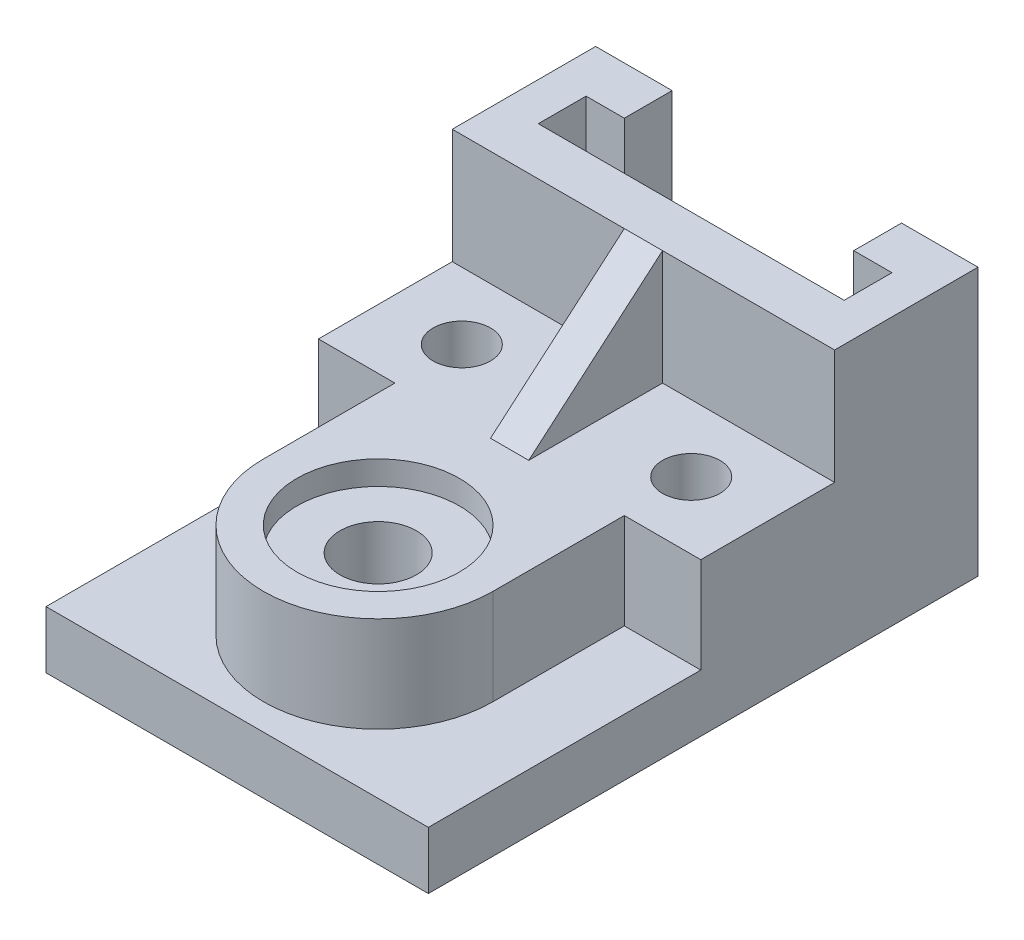
ISO-10303-21;
HEADER;
FILE_DESCRIPTION(('STEP AP214'),'2;1');
FILE_NAME('part.step','',(''),(''),'','','');
FILE_SCHEMA(('AUTOMOTIVE_DESIGN { 1 0 10303 214 1 1 1 1 }'));
ENDSEC;
DATA;
#1=APPLICATION_CONTEXT('core data for automotive mechanical design processes');
#2=APPLICATION_PROTOCOL_DEFINITION('international standard','automotive_design',2000,#1);
#3=PRODUCT_CONTEXT('',#1,'mechanical');
#4=PRODUCT('Part','Part','',(#3));
#5=PRODUCT_RELATED_PRODUCT_CATEGORY('part','',(#4));
#6=PRODUCT_DEFINITION_FORMATION('','',#4);
#7=PRODUCT_DEFINITION_CONTEXT('part definition',#1,'design');
#8=PRODUCT_DEFINITION('design','',#6,#7);
#9=PRODUCT_DEFINITION_SHAPE('','',#8);
#10=(LENGTH_UNIT() NAMED_UNIT(*) SI_UNIT(.MILLI.,.METRE.));
#11=(NAMED_UNIT(*) PLANE_ANGLE_UNIT() SI_UNIT($,.RADIAN.));
#12=(NAMED_UNIT(*) SI_UNIT($,.STERADIAN.) SOLID_ANGLE_UNIT());
#13=UNCERTAINTY_MEASURE_WITH_UNIT(LENGTH_MEASURE(1.E-05),#10,'distance_accuracy_value','');
#14=(GEOMETRIC_REPRESENTATION_CONTEXT(3) GLOBAL_UNCERTAINTY_ASSIGNED_CONTEXT((#13)) GLOBAL_UNIT_ASSIGNED_CONTEXT((#10,
#11,#12)) REPRESENTATION_CONTEXT('',''));
#15=CARTESIAN_POINT('',(0.,0.,0.));
#16=DIRECTION('',(0.,0.,1.));
#17=DIRECTION('',(1.,0.,0.));
#18=AXIS2_PLACEMENT_3D('',#15,#16,#17);
#19=CARTESIAN_POINT('',(-40.,56.,-27.5));
#20=DIRECTION('',(0.,0.,-1.));
#21=DIRECTION('',(-1.,0.,0.));
#22=AXIS2_PLACEMENT_3D('',#19,#20,#21);
#23=PLANE('',#22);
#24=DIRECTION('',(0.,-1.,0.));
#25=VECTOR('',#24,1.);
#26=CARTESIAN_POINT('',(-4.,56.,-27.5));
#27=LINE('',#26,#25);
#28=CARTESIAN_POINT('',(-4.,56.,-27.5));
#29=VERTEX_POINT('',#28);
#30=CARTESIAN_POINT('',(-4.,32.,-27.5));
#31=VERTEX_POINT('',#30);
#32=EDGE_CURVE('E57',#29,#31,#27,.T.);
#33=ORIENTED_EDGE('',*,*,#32,.F.);
#34=DIRECTION('',(1.,0.,0.));
#35=VECTOR('',#34,1.);
#36=CARTESIAN_POINT('',(-40.,56.,-27.5));
#37=LINE('',#36,#35);
#38=CARTESIAN_POINT('',(-40.,56.,-27.5));
#39=VERTEX_POINT('',#38);
#40=EDGE_CURVE('E220',#39,#29,#37,.T.);
#41=ORIENTED_EDGE('',*,*,#40,.F.);
#42=DIRECTION('',(0.,-1.,0.));
#43=VECTOR('',#42,1.);
#44=CARTESIAN_POINT('',(-40.,56.,-27.5));
#45=LINE('',#44,#43);
#46=CARTESIAN_POINT('',(-40.,32.,-27.5));
#47=VERTEX_POINT('',#46);
#48=EDGE_CURVE('E245',#39,#47,#45,.T.);
#49=ORIENTED_EDGE('',*,*,#48,.T.);
#50=DIRECTION('',(-1.,0.,0.));
#51=VECTOR('',#50,1.);
#52=CARTESIAN_POINT('',(-40.,32.,-27.5));
#53=LINE('',#52,#51);
#54=EDGE_CURVE('E218',#31,#47,#53,.T.);
#55=ORIENTED_EDGE('',*,*,#54,.F.);
#56=EDGE_LOOP('',(#33,#41,#49,#55));
#57=FACE_BOUND('',#56,.T.);
#58=ADVANCED_FACE('F41',(#57),#23,.F.);
#59=CARTESIAN_POINT('',(-40.,12.,-57.5));
#60=DIRECTION('',(0.,0.,1.));
#61=DIRECTION('',(1.,0.,0.));
#62=AXIS2_PLACEMENT_3D('',#59,#60,#61);
#63=PLANE('',#62);
#64=DIRECTION('',(-1.,0.,0.));
#65=VECTOR('',#64,1.);
#66=CARTESIAN_POINT('',(-40.,0.,-57.5));
#67=LINE('',#66,#65);
#68=CARTESIAN_POINT('',(40.,0.,-57.5));
#69=VERTEX_POINT('',#68);
#70=CARTESIAN_POINT('',(24.,0.,-57.5));
#71=VERTEX_POINT('',#70);
#72=EDGE_CURVE('E260',#69,#71,#67,.T.);
#73=ORIENTED_EDGE('',*,*,#72,.T.);
#74=DIRECTION('',(0.,1.,0.));
#75=VECTOR('',#74,1.);
#76=CARTESIAN_POINT('',(24.,0.,-57.5));
#77=LINE('',#76,#75);
#78=CARTESIAN_POINT('',(24.,56.,-57.5));
#79=VERTEX_POINT('',#78);
#80=EDGE_CURVE('E348',#71,#79,#77,.T.);
#81=ORIENTED_EDGE('',*,*,#80,.T.);
#82=DIRECTION('',(-1.,0.,0.));
#83=VECTOR('',#82,1.);
#84=CARTESIAN_POINT('',(-40.,56.,-57.5));
#85=LINE('',#84,#83);
#86=CARTESIAN_POINT('',(40.,56.,-57.5));
#87=VERTEX_POINT('',#86);
#88=EDGE_CURVE('E237',#87,#79,#85,.T.);
#89=ORIENTED_EDGE('',*,*,#88,.F.);
#90=DIRECTION('',(0.,-1.,0.));
#91=VECTOR('',#90,1.);
#92=CARTESIAN_POINT('',(40.,12.,-57.5));
#93=LINE('',#92,#91);
#94=EDGE_CURVE('E11',#87,#69,#93,.T.);
#95=ORIENTED_EDGE('',*,*,#94,.T.);
#96=EDGE_LOOP('',(#73,#81,#89,#95));
#97=FACE_BOUND('',#96,.T.);
#98=ADVANCED_FACE('F378',(#97),#63,.F.);
#99=CARTESIAN_POINT('',(0.,12.,0.));
#100=DIRECTION('',(0.,-1.,0.));
#101=DIRECTION('',(0.,0.,-1.));
#102=AXIS2_PLACEMENT_3D('',#99,#100,#101);
#103=PLANE('',#102);
#104=DIRECTION('',(1.,0.,0.));
#105=VECTOR('',#104,1.);
#106=CARTESIAN_POINT('',(-40.,12.,0.499999999999997));
#107=LINE('',#106,#105);
#108=CARTESIAN_POINT('',(-40.,12.,0.499999999999997));
#109=VERTEX_POINT('',#108);
#110=CARTESIAN_POINT('',(-24.,12.,0.499999999999997));
#111=VERTEX_POINT('',#110);
#112=EDGE_CURVE('E299',#109,#111,#107,.T.);
#113=ORIENTED_EDGE('',*,*,#112,.F.);
#114=DIRECTION('',(0.,0.,1.));
#115=VECTOR('',#114,1.);
#116=CARTESIAN_POINT('',(-40.,12.,57.5));
#117=LINE('',#116,#115);
#118=CARTESIAN_POINT('',(-40.,12.,57.5));
#119=VERTEX_POINT('',#118);
#120=EDGE_CURVE('E246',#109,#119,#117,.T.);
#121=ORIENTED_EDGE('',*,*,#120,.T.);
#122=DIRECTION('',(1.,0.,0.));
#123=VECTOR('',#122,1.);
#124=CARTESIAN_POINT('',(-40.,12.,57.5));
#125=LINE('',#124,#123);
#126=CARTESIAN_POINT('',(40.,12.,57.5));
#127=VERTEX_POINT('',#126);
#128=EDGE_CURVE('E253',#119,#127,#125,.T.);
#129=ORIENTED_EDGE('',*,*,#128,.T.);
#130=DIRECTION('',(0.,0.,-1.));
#131=VECTOR('',#130,1.);
#132=CARTESIAN_POINT('',(40.,12.,57.5));
#133=LINE('',#132,#131);
#134=CARTESIAN_POINT('',(40.,12.,0.499999999999997));
#135=VERTEX_POINT('',#134);
#136=EDGE_CURVE('E242',#127,#135,#133,.T.);
#137=ORIENTED_EDGE('',*,*,#136,.T.);
#138=DIRECTION('',(1.,0.,0.));
#139=VECTOR('',#138,1.);
#140=CARTESIAN_POINT('',(24.,12.,0.499999999999997));
#141=LINE('',#140,#139);
#142=CARTESIAN_POINT('',(24.,12.,0.499999999999997));
#143=VERTEX_POINT('',#142);
#144=EDGE_CURVE('E300',#143,#135,#141,.T.);
#145=ORIENTED_EDGE('',*,*,#144,.F.);
#146=DIRECTION('',(0.,0.,-1.));
#147=VECTOR('',#146,1.);
#148=CARTESIAN_POINT('',(24.,12.,28.));
#149=LINE('',#148,#147);
#150=CARTESIAN_POINT('',(24.,12.,28.));
#151=VERTEX_POINT('',#150);
#152=EDGE_CURVE('E705',#151,#143,#149,.T.);
#153=ORIENTED_EDGE('',*,*,#152,.F.);
#154=CARTESIAN_POINT('',(0.,12.,28.));
#155=DIRECTION('',(0.,1.,0.));
#156=DIRECTION('',(0.,0.,1.));
#157=AXIS2_PLACEMENT_3D('',#154,#155,#156);
#158=CIRCLE('',#157,24.);
#159=CARTESIAN_POINT('',(-24.,12.,28.));
#160=VERTEX_POINT('',#159);
#161=EDGE_CURVE('E697',#160,#151,#158,.T.);
#162=ORIENTED_EDGE('',*,*,#161,.F.);
#163=DIRECTION('',(0.,0.,1.));
#164=VECTOR('',#163,1.);
#165=CARTESIAN_POINT('',(-24.,12.,28.));
#166=LINE('',#165,#164);
#167=EDGE_CURVE('E696',#111,#160,#166,.T.);
#168=ORIENTED_EDGE('',*,*,#167,.F.);
#169=EDGE_LOOP('',(#113,#121,#129,#137,#145,#153,#162,#168));
#170=FACE_BOUND('',#169,.T.);
#171=ADVANCED_FACE('F293',(#170),#103,.F.);
#172=CARTESIAN_POINT('',(40.,12.,57.5));
#173=DIRECTION('',(-1.,0.,0.));
#174=DIRECTION('',(0.,0.,1.));
#175=AXIS2_PLACEMENT_3D('',#172,#173,#174);
#176=PLANE('',#175);
#177=DIRECTION('',(0.,0.,-1.));
#178=VECTOR('',#177,1.);
#179=CARTESIAN_POINT('',(40.,0.,57.5));
#180=LINE('',#179,#178);
#181=CARTESIAN_POINT('',(40.,0.,57.5));
#182=VERTEX_POINT('',#181);
#183=EDGE_CURVE('E244',#182,#69,#180,.T.);
#184=ORIENTED_EDGE('',*,*,#183,.T.);
#185=ORIENTED_EDGE('',*,*,#94,.F.);
#186=DIRECTION('',(0.,0.,-1.));
#187=VECTOR('',#186,1.);
#188=CARTESIAN_POINT('',(40.,56.,-57.5));
#189=LINE('',#188,#187);
#190=CARTESIAN_POINT('',(40.,56.,-27.5));
#191=VERTEX_POINT('',#190);
#192=EDGE_CURVE('E230',#191,#87,#189,.T.);
#193=ORIENTED_EDGE('',*,*,#192,.F.);
#194=DIRECTION('',(0.,-1.,0.));
#195=VECTOR('',#194,1.);
#196=CARTESIAN_POINT('',(40.,56.,-27.5));
#197=LINE('',#196,#195);
#198=CARTESIAN_POINT('',(40.,32.,-27.5));
#199=VERTEX_POINT('',#198);
#200=EDGE_CURVE('E239',#191,#199,#197,.T.);
#201=ORIENTED_EDGE('',*,*,#200,.T.);
#202=DIRECTION('',(0.,0.,-1.));
#203=VECTOR('',#202,1.);
#204=CARTESIAN_POINT('',(40.,32.,-27.5));
#205=LINE('',#204,#203);
#206=CARTESIAN_POINT('',(40.,32.,0.499999999999997));
#207=VERTEX_POINT('',#206);
#208=EDGE_CURVE('E691',#207,#199,#205,.T.);
#209=ORIENTED_EDGE('',*,*,#208,.F.);
#210=DIRECTION('',(0.,-1.,0.));
#211=VECTOR('',#210,1.);
#212=CARTESIAN_POINT('',(40.,32.,0.499999999999997));
#213=LINE('',#212,#211);
#214=EDGE_CURVE('E292',#207,#135,#213,.T.);
#215=ORIENTED_EDGE('',*,*,#214,.T.);
#216=ORIENTED_EDGE('',*,*,#136,.F.);
#217=DIRECTION('',(0.,-1.,0.));
#218=VECTOR('',#217,1.);
#219=CARTESIAN_POINT('',(40.,12.,57.5));
#220=LINE('',#219,#218);
#221=EDGE_CURVE('E251',#127,#182,#220,.T.);
#222=ORIENTED_EDGE('',*,*,#221,.T.);
#223=EDGE_LOOP('',(#184,#185,#193,#201,#209,#215,#216,#222));
#224=FACE_BOUND('',#223,.T.);
#225=ADVANCED_FACE('F43',(#224),#176,.F.);
#226=CARTESIAN_POINT('',(-24.,56.,-57.5));
#227=VERTEX_POINT('',#226);
#228=CARTESIAN_POINT('',(-40.,56.,-57.5));
#229=VERTEX_POINT('',#228);
#230=EDGE_CURVE('E233',#227,#229,#85,.T.);
#231=ORIENTED_EDGE('',*,*,#230,.F.);
#232=DIRECTION('',(0.,1.,0.));
#233=VECTOR('',#232,1.);
#234=CARTESIAN_POINT('',(-24.,0.,-57.5));
#235=LINE('',#234,#233);
#236=CARTESIAN_POINT('',(-24.,0.,-57.5));
#237=VERTEX_POINT('',#236);
#238=EDGE_CURVE('E64',#237,#227,#235,.T.);
#239=ORIENTED_EDGE('',*,*,#238,.F.);
#240=CARTESIAN_POINT('',(-40.,0.,-57.5));
#241=VERTEX_POINT('',#240);
#242=EDGE_CURVE('E258',#237,#241,#67,.T.);
#243=ORIENTED_EDGE('',*,*,#242,.T.);
#244=DIRECTION('',(0.,-1.,0.));
#245=VECTOR('',#244,1.);
#246=CARTESIAN_POINT('',(-40.,12.,-57.5));
#247=LINE('',#246,#245);
#248=EDGE_CURVE('E47',#229,#241,#247,.T.);
#249=ORIENTED_EDGE('',*,*,#248,.F.);
#250=EDGE_LOOP('',(#231,#239,#243,#249));
#251=FACE_BOUND('',#250,.T.);
#252=ADVANCED_FACE('F376',(#251),#63,.F.);
#253=CARTESIAN_POINT('',(-40.,12.,57.5));
#254=DIRECTION('',(1.,0.,0.));
#255=DIRECTION('',(0.,0.,-1.));
#256=AXIS2_PLACEMENT_3D('',#253,#254,#255);
#257=PLANE('',#256);
#258=ORIENTED_EDGE('',*,*,#120,.F.);
#259=DIRECTION('',(0.,-1.,0.));
#260=VECTOR('',#259,1.);
#261=CARTESIAN_POINT('',(-40.,32.,0.499999999999997));
#262=LINE('',#261,#260);
#263=CARTESIAN_POINT('',(-40.,32.,0.499999999999997));
#264=VERTEX_POINT('',#263);
#265=EDGE_CURVE('E305',#264,#109,#262,.T.);
#266=ORIENTED_EDGE('',*,*,#265,.F.);
#267=DIRECTION('',(0.,0.,1.));
#268=VECTOR('',#267,1.);
#269=CARTESIAN_POINT('',(-40.,32.,-27.5));
#270=LINE('',#269,#268);
#271=EDGE_CURVE('E304',#47,#264,#270,.T.);
#272=ORIENTED_EDGE('',*,*,#271,.F.);
#273=ORIENTED_EDGE('',*,*,#48,.F.);
#274=DIRECTION('',(0.,0.,1.));
#275=VECTOR('',#274,1.);
#276=CARTESIAN_POINT('',(-40.,56.,-57.5));
#277=LINE('',#276,#275);
#278=EDGE_CURVE('E223',#229,#39,#277,.T.);
#279=ORIENTED_EDGE('',*,*,#278,.F.);
#280=ORIENTED_EDGE('',*,*,#248,.T.);
#281=DIRECTION('',(0.,0.,1.));
#282=VECTOR('',#281,1.);
#283=CARTESIAN_POINT('',(-40.,0.,57.5));
#284=LINE('',#283,#282);
#285=CARTESIAN_POINT('',(-40.,0.,57.5));
#286=VERTEX_POINT('',#285);
#287=EDGE_CURVE('E257',#241,#286,#284,.T.);
#288=ORIENTED_EDGE('',*,*,#287,.T.);
#289=DIRECTION('',(0.,-1.,0.));
#290=VECTOR('',#289,1.);
#291=CARTESIAN_POINT('',(-40.,12.,57.5));
#292=LINE('',#291,#290);
#293=EDGE_CURVE('E264',#119,#286,#292,.T.);
#294=ORIENTED_EDGE('',*,*,#293,.F.);
#295=EDGE_LOOP('',(#258,#266,#272,#273,#279,#280,#288,#294));
#296=FACE_BOUND('',#295,.T.);
#297=ADVANCED_FACE('F275',(#296),#257,.F.);
#298=CARTESIAN_POINT('',(-40.,12.,57.5));
#299=DIRECTION('',(0.,0.,-1.));
#300=DIRECTION('',(-1.,0.,0.));
#301=AXIS2_PLACEMENT_3D('',#298,#299,#300);
#302=PLANE('',#301);
#303=DIRECTION('',(1.,0.,0.));
#304=VECTOR('',#303,1.);
#305=CARTESIAN_POINT('',(-40.,0.,57.5));
#306=LINE('',#305,#304);
#307=EDGE_CURVE('E249',#286,#182,#306,.T.);
#308=ORIENTED_EDGE('',*,*,#307,.T.);
#309=ORIENTED_EDGE('',*,*,#221,.F.);
#310=ORIENTED_EDGE('',*,*,#128,.F.);
#311=ORIENTED_EDGE('',*,*,#293,.T.);
#312=EDGE_LOOP('',(#308,#309,#310,#311));
#313=FACE_BOUND('',#312,.T.);
#314=ADVANCED_FACE('F284',(#313),#302,.F.);
#315=CARTESIAN_POINT('',(0.,0.,0.));
#316=DIRECTION('',(0.,-1.,0.));
#317=DIRECTION('',(0.,0.,-1.));
#318=AXIS2_PLACEMENT_3D('',#315,#316,#317);
#319=PLANE('',#318);
#320=DIRECTION('',(1.,0.,0.));
#321=VECTOR('',#320,1.);
#322=CARTESIAN_POINT('',(-32.,0.,-37.5));
#323=LINE('',#322,#321);
#324=CARTESIAN_POINT('',(-32.,0.,-37.5));
#325=VERTEX_POINT('',#324);
#326=CARTESIAN_POINT('',(32.,0.,-37.5));
#327=VERTEX_POINT('',#326);
#328=EDGE_CURVE('E324',#325,#327,#323,.T.);
#329=ORIENTED_EDGE('',*,*,#328,.T.);
#330=DIRECTION('',(0.,0.,-1.));
#331=VECTOR('',#330,1.);
#332=CARTESIAN_POINT('',(32.,0.,-37.5));
#333=LINE('',#332,#331);
#334=CARTESIAN_POINT('',(32.,0.,-47.5));
#335=VERTEX_POINT('',#334);
#336=EDGE_CURVE('E330',#327,#335,#333,.T.);
#337=ORIENTED_EDGE('',*,*,#336,.T.);
#338=DIRECTION('',(-1.,0.,0.));
#339=VECTOR('',#338,1.);
#340=CARTESIAN_POINT('',(32.,0.,-47.5));
#341=LINE('',#340,#339);
#342=CARTESIAN_POINT('',(24.,0.,-47.5));
#343=VERTEX_POINT('',#342);
#344=EDGE_CURVE('E329',#335,#343,#341,.T.);
#345=ORIENTED_EDGE('',*,*,#344,.T.);
#346=DIRECTION('',(0.,0.,-1.));
#347=VECTOR('',#346,1.);
#348=CARTESIAN_POINT('',(24.,0.,-47.5));
#349=LINE('',#348,#347);
#350=EDGE_CURVE('E334',#343,#71,#349,.T.);
#351=ORIENTED_EDGE('',*,*,#350,.T.);
#352=ORIENTED_EDGE('',*,*,#72,.F.);
#353=ORIENTED_EDGE('',*,*,#183,.F.);
#354=ORIENTED_EDGE('',*,*,#307,.F.);
#355=ORIENTED_EDGE('',*,*,#287,.F.);
#356=ORIENTED_EDGE('',*,*,#242,.F.);
#357=DIRECTION('',(0.,0.,1.));
#358=VECTOR('',#357,1.);
#359=CARTESIAN_POINT('',(-24.,0.,-57.5));
#360=LINE('',#359,#358);
#361=CARTESIAN_POINT('',(-24.,0.,-47.5));
#362=VERTEX_POINT('',#361);
#363=EDGE_CURVE('E316',#237,#362,#360,.T.);
#364=ORIENTED_EDGE('',*,*,#363,.T.);
#365=DIRECTION('',(-1.,0.,0.));
#366=VECTOR('',#365,1.);
#367=CARTESIAN_POINT('',(-24.,0.,-47.5));
#368=LINE('',#367,#366);
#369=CARTESIAN_POINT('',(-32.,0.,-47.5));
#370=VERTEX_POINT('',#369);
#371=EDGE_CURVE('E318',#362,#370,#368,.T.);
#372=ORIENTED_EDGE('',*,*,#371,.T.);
#373=DIRECTION('',(0.,0.,1.));
#374=VECTOR('',#373,1.);
#375=CARTESIAN_POINT('',(-32.,0.,-47.5));
#376=LINE('',#375,#374);
#377=EDGE_CURVE('E325',#370,#325,#376,.T.);
#378=ORIENTED_EDGE('',*,*,#377,.T.);
#379=EDGE_LOOP('',(#329,#337,#345,#351,#352,#353,#354,#355,#356,#364,#372,#378));
#380=FACE_BOUND('',#379,.T.);
#381=ADVANCED_FACE('F276',(#380),#319,.T.);
#382=CARTESIAN_POINT('',(4.,56.,-27.5));
#383=VERTEX_POINT('',#382);
#384=EDGE_CURVE('E226',#383,#191,#37,.T.);
#385=ORIENTED_EDGE('',*,*,#384,.F.);
#386=DIRECTION('',(0.,-1.,0.));
#387=VECTOR('',#386,1.);
#388=CARTESIAN_POINT('',(4.,56.,-27.5));
#389=LINE('',#388,#387);
#390=CARTESIAN_POINT('',(4.,32.,-27.5));
#391=VERTEX_POINT('',#390);
#392=EDGE_CURVE('E408',#383,#391,#389,.T.);
#393=ORIENTED_EDGE('',*,*,#392,.T.);
#394=EDGE_CURVE('E694',#199,#391,#53,.T.);
#395=ORIENTED_EDGE('',*,*,#394,.F.);
#396=ORIENTED_EDGE('',*,*,#200,.F.);
#397=EDGE_LOOP('',(#385,#393,#395,#396));
#398=FACE_BOUND('',#397,.T.);
#399=ADVANCED_FACE('F386',(#398),#23,.F.);
#400=CARTESIAN_POINT('',(0.,56.,0.));
#401=DIRECTION('',(0.,1.,0.));
#402=DIRECTION('',(0.,0.,1.));
#403=AXIS2_PLACEMENT_3D('',#400,#401,#402);
#404=PLANE('',#403);
#405=DIRECTION('',(0.,0.,-1.));
#406=VECTOR('',#405,1.);
#407=CARTESIAN_POINT('',(32.,56.,-37.5));
#408=LINE('',#407,#406);
#409=CARTESIAN_POINT('',(32.,56.,-37.5));
#410=VERTEX_POINT('',#409);
#411=CARTESIAN_POINT('',(32.,56.,-47.5));
#412=VERTEX_POINT('',#411);
#413=EDGE_CURVE('E341',#410,#412,#408,.T.);
#414=ORIENTED_EDGE('',*,*,#413,.F.);
#415=DIRECTION('',(1.,0.,0.));
#416=VECTOR('',#415,1.);
#417=CARTESIAN_POINT('',(-32.,56.,-37.5));
#418=LINE('',#417,#416);
#419=CARTESIAN_POINT('',(-32.,56.,-37.5));
#420=VERTEX_POINT('',#419);
#421=EDGE_CURVE('E343',#420,#410,#418,.T.);
#422=ORIENTED_EDGE('',*,*,#421,.F.);
#423=DIRECTION('',(0.,0.,1.));
#424=VECTOR('',#423,1.);
#425=CARTESIAN_POINT('',(-32.,56.,-47.5));
#426=LINE('',#425,#424);
#427=CARTESIAN_POINT('',(-32.,56.,-47.5));
#428=VERTEX_POINT('',#427);
#429=EDGE_CURVE('E336',#428,#420,#426,.T.);
#430=ORIENTED_EDGE('',*,*,#429,.F.);
#431=DIRECTION('',(-1.,0.,0.));
#432=VECTOR('',#431,1.);
#433=CARTESIAN_POINT('',(-24.,56.,-47.5));
#434=LINE('',#433,#432);
#435=CARTESIAN_POINT('',(-24.,56.,-47.5));
#436=VERTEX_POINT('',#435);
#437=EDGE_CURVE('E310',#436,#428,#434,.T.);
#438=ORIENTED_EDGE('',*,*,#437,.F.);
#439=DIRECTION('',(0.,0.,1.));
#440=VECTOR('',#439,1.);
#441=CARTESIAN_POINT('',(-24.,56.,-57.5));
#442=LINE('',#441,#440);
#443=EDGE_CURVE('E308',#227,#436,#442,.T.);
#444=ORIENTED_EDGE('',*,*,#443,.F.);
#445=ORIENTED_EDGE('',*,*,#230,.T.);
#446=ORIENTED_EDGE('',*,*,#278,.T.);
#447=ORIENTED_EDGE('',*,*,#40,.T.);
#448=DIRECTION('',(1.,0.,0.));
#449=VECTOR('',#448,1.);
#450=CARTESIAN_POINT('',(0.,56.,-27.5));
#451=LINE('',#450,#449);
#452=EDGE_CURVE('E200',#29,#383,#451,.T.);
#453=ORIENTED_EDGE('',*,*,#452,.T.);
#454=ORIENTED_EDGE('',*,*,#384,.T.);
#455=ORIENTED_EDGE('',*,*,#192,.T.);
#456=ORIENTED_EDGE('',*,*,#88,.T.);
#457=DIRECTION('',(0.,0.,-1.));
#458=VECTOR('',#457,1.);
#459=CARTESIAN_POINT('',(24.,56.,-47.5));
#460=LINE('',#459,#458);
#461=CARTESIAN_POINT('',(24.,56.,-47.5));
#462=VERTEX_POINT('',#461);
#463=EDGE_CURVE('E317',#462,#79,#460,.T.);
#464=ORIENTED_EDGE('',*,*,#463,.F.);
#465=DIRECTION('',(-1.,0.,0.));
#466=VECTOR('',#465,1.);
#467=CARTESIAN_POINT('',(32.,56.,-47.5));
#468=LINE('',#467,#466);
#469=EDGE_CURVE('E347',#412,#462,#468,.T.);
#470=ORIENTED_EDGE('',*,*,#469,.F.);
#471=EDGE_LOOP('',(#414,#422,#430,#438,#444,#445,#446,#447,#453,#454,#455,#456,#464,#470));
#472=FACE_BOUND('',#471,.T.);
#473=ADVANCED_FACE('F224',(#472),#404,.T.);
#474=CARTESIAN_POINT('',(24.,0.,-47.5));
#475=DIRECTION('',(1.,0.,0.));
#476=DIRECTION('',(0.,0.,-1.));
#477=AXIS2_PLACEMENT_3D('',#474,#475,#476);
#478=PLANE('',#477);
#479=ORIENTED_EDGE('',*,*,#463,.T.);
#480=ORIENTED_EDGE('',*,*,#80,.F.);
#481=ORIENTED_EDGE('',*,*,#350,.F.);
#482=DIRECTION('',(0.,1.,0.));
#483=VECTOR('',#482,1.);
#484=CARTESIAN_POINT('',(24.,0.,-47.5));
#485=LINE('',#484,#483);
#486=EDGE_CURVE('E351',#343,#462,#485,.T.);
#487=ORIENTED_EDGE('',*,*,#486,.T.);
#488=EDGE_LOOP('',(#479,#480,#481,#487));
#489=FACE_BOUND('',#488,.T.);
#490=ADVANCED_FACE('F402',(#489),#478,.F.);
#491=CARTESIAN_POINT('',(32.,0.,-47.5));
#492=DIRECTION('',(0.,0.,-1.));
#493=DIRECTION('',(-1.,0.,0.));
#494=AXIS2_PLACEMENT_3D('',#491,#492,#493);
#495=PLANE('',#494);
#496=ORIENTED_EDGE('',*,*,#469,.T.);
#497=ORIENTED_EDGE('',*,*,#486,.F.);
#498=ORIENTED_EDGE('',*,*,#344,.F.);
#499=DIRECTION('',(0.,1.,0.));
#500=VECTOR('',#499,1.);
#501=CARTESIAN_POINT('',(32.,0.,-47.5));
#502=LINE('',#501,#500);
#503=EDGE_CURVE('E352',#335,#412,#502,.T.);
#504=ORIENTED_EDGE('',*,*,#503,.T.);
#505=EDGE_LOOP('',(#496,#497,#498,#504));
#506=FACE_BOUND('',#505,.T.);
#507=ADVANCED_FACE('F418',(#506),#495,.F.);
#508=CARTESIAN_POINT('',(32.,0.,-37.5));
#509=DIRECTION('',(1.,0.,0.));
#510=DIRECTION('',(0.,0.,-1.));
#511=AXIS2_PLACEMENT_3D('',#508,#509,#510);
#512=PLANE('',#511);
#513=ORIENTED_EDGE('',*,*,#413,.T.);
#514=ORIENTED_EDGE('',*,*,#503,.F.);
#515=ORIENTED_EDGE('',*,*,#336,.F.);
#516=DIRECTION('',(0.,1.,0.));
#517=VECTOR('',#516,1.);
#518=CARTESIAN_POINT('',(32.,0.,-37.5));
#519=LINE('',#518,#517);
#520=EDGE_CURVE('E360',#327,#410,#519,.T.);
#521=ORIENTED_EDGE('',*,*,#520,.T.);
#522=EDGE_LOOP('',(#513,#514,#515,#521));
#523=FACE_BOUND('',#522,.T.);
#524=ADVANCED_FACE('F420',(#523),#512,.F.);
#525=CARTESIAN_POINT('',(-32.,0.,-37.5));
#526=DIRECTION('',(0.,0.,1.));
#527=DIRECTION('',(1.,0.,0.));
#528=AXIS2_PLACEMENT_3D('',#525,#526,#527);
#529=PLANE('',#528);
#530=ORIENTED_EDGE('',*,*,#520,.F.);
#531=ORIENTED_EDGE('',*,*,#328,.F.);
#532=DIRECTION('',(0.,1.,0.));
#533=VECTOR('',#532,1.);
#534=CARTESIAN_POINT('',(-32.,0.,-37.5));
#535=LINE('',#534,#533);
#536=EDGE_CURVE('E357',#325,#420,#535,.T.);
#537=ORIENTED_EDGE('',*,*,#536,.T.);
#538=ORIENTED_EDGE('',*,*,#421,.T.);
#539=EDGE_LOOP('',(#530,#531,#537,#538));
#540=FACE_BOUND('',#539,.T.);
#541=ADVANCED_FACE('F425',(#540),#529,.F.);
#542=CARTESIAN_POINT('',(-32.,0.,-47.5));
#543=DIRECTION('',(-1.,0.,0.));
#544=DIRECTION('',(0.,0.,1.));
#545=AXIS2_PLACEMENT_3D('',#542,#543,#544);
#546=PLANE('',#545);
#547=ORIENTED_EDGE('',*,*,#429,.T.);
#548=ORIENTED_EDGE('',*,*,#536,.F.);
#549=ORIENTED_EDGE('',*,*,#377,.F.);
#550=DIRECTION('',(0.,1.,0.));
#551=VECTOR('',#550,1.);
#552=CARTESIAN_POINT('',(-32.,0.,-47.5));
#553=LINE('',#552,#551);
#554=EDGE_CURVE('E362',#370,#428,#553,.T.);
#555=ORIENTED_EDGE('',*,*,#554,.T.);
#556=EDGE_LOOP('',(#547,#548,#549,#555));
#557=FACE_BOUND('',#556,.T.);
#558=ADVANCED_FACE('F373',(#557),#546,.F.);
#559=CARTESIAN_POINT('',(-24.,0.,-47.5));
#560=DIRECTION('',(0.,0.,-1.));
#561=DIRECTION('',(-1.,0.,0.));
#562=AXIS2_PLACEMENT_3D('',#559,#560,#561);
#563=PLANE('',#562);
#564=ORIENTED_EDGE('',*,*,#437,.T.);
#565=ORIENTED_EDGE('',*,*,#554,.F.);
#566=ORIENTED_EDGE('',*,*,#371,.F.);
#567=DIRECTION('',(0.,1.,0.));
#568=VECTOR('',#567,1.);
#569=CARTESIAN_POINT('',(-24.,0.,-47.5));
#570=LINE('',#569,#568);
#571=EDGE_CURVE('E365',#362,#436,#570,.T.);
#572=ORIENTED_EDGE('',*,*,#571,.T.);
#573=EDGE_LOOP('',(#564,#565,#566,#572));
#574=FACE_BOUND('',#573,.T.);
#575=ADVANCED_FACE('F370',(#574),#563,.F.);
#576=CARTESIAN_POINT('',(-24.,0.,-57.5));
#577=DIRECTION('',(-1.,0.,0.));
#578=DIRECTION('',(0.,0.,1.));
#579=AXIS2_PLACEMENT_3D('',#576,#577,#578);
#580=PLANE('',#579);
#581=ORIENTED_EDGE('',*,*,#443,.T.);
#582=ORIENTED_EDGE('',*,*,#571,.F.);
#583=ORIENTED_EDGE('',*,*,#363,.F.);
#584=ORIENTED_EDGE('',*,*,#238,.T.);
#585=EDGE_LOOP('',(#581,#582,#583,#584));
#586=FACE_BOUND('',#585,.T.);
#587=ADVANCED_FACE('F367',(#586),#580,.F.);
#588=CARTESIAN_POINT('',(0.,32.,28.));
#589=DIRECTION('',(0.,1.,0.));
#590=DIRECTION('',(0.,0.,1.));
#591=AXIS2_PLACEMENT_3D('',#588,#589,#590);
#592=PLANE('',#591);
#593=DIRECTION('',(0.,0.,-1.));
#594=VECTOR('',#593,1.);
#595=CARTESIAN_POINT('',(4.,32.,28.));
#596=LINE('',#595,#594);
#597=CARTESIAN_POINT('',(4.,32.,0.499999999999994));
#598=VERTEX_POINT('',#597);
#599=EDGE_CURVE('E219',#598,#391,#596,.T.);
#600=ORIENTED_EDGE('',*,*,#599,.F.);
#601=DIRECTION('',(1.,0.,0.));
#602=VECTOR('',#601,1.);
#603=CARTESIAN_POINT('',(0.,32.,0.49999999999999));
#604=LINE('',#603,#602);
#605=CARTESIAN_POINT('',(-4.,32.,0.499999999999994));
#606=VERTEX_POINT('',#605);
#607=EDGE_CURVE('E207',#606,#598,#604,.T.);
#608=ORIENTED_EDGE('',*,*,#607,.F.);
#609=DIRECTION('',(0.,0.,-1.));
#610=VECTOR('',#609,1.);
#611=CARTESIAN_POINT('',(-4.,32.,28.));
#612=LINE('',#611,#610);
#613=EDGE_CURVE('E215',#606,#31,#612,.T.);
#614=ORIENTED_EDGE('',*,*,#613,.T.);
#615=ORIENTED_EDGE('',*,*,#54,.T.);
#616=ORIENTED_EDGE('',*,*,#271,.T.);
#617=DIRECTION('',(1.,0.,0.));
#618=VECTOR('',#617,1.);
#619=CARTESIAN_POINT('',(-40.,32.,0.499999999999997));
#620=LINE('',#619,#618);
#621=CARTESIAN_POINT('',(-24.,32.,0.499999999999997));
#622=VERTEX_POINT('',#621);
#623=EDGE_CURVE('E681',#264,#622,#620,.T.);
#624=ORIENTED_EDGE('',*,*,#623,.T.);
#625=DIRECTION('',(0.,0.,1.));
#626=VECTOR('',#625,1.);
#627=CARTESIAN_POINT('',(-24.,32.,28.));
#628=LINE('',#627,#626);
#629=CARTESIAN_POINT('',(-24.,32.,28.));
#630=VERTEX_POINT('',#629);
#631=EDGE_CURVE('E682',#622,#630,#628,.T.);
#632=ORIENTED_EDGE('',*,*,#631,.T.);
#633=CARTESIAN_POINT('',(0.,32.,28.));
#634=DIRECTION('',(0.,1.,0.));
#635=DIRECTION('',(0.,0.,1.));
#636=AXIS2_PLACEMENT_3D('',#633,#634,#635);
#637=CIRCLE('',#636,24.);
#638=CARTESIAN_POINT('',(24.,32.,28.));
#639=VERTEX_POINT('',#638);
#640=EDGE_CURVE('E690',#630,#639,#637,.T.);
#641=ORIENTED_EDGE('',*,*,#640,.T.);
#642=DIRECTION('',(0.,0.,-1.));
#643=VECTOR('',#642,1.);
#644=CARTESIAN_POINT('',(24.,32.,28.));
#645=LINE('',#644,#643);
#646=CARTESIAN_POINT('',(24.,32.,0.499999999999997));
#647=VERTEX_POINT('',#646);
#648=EDGE_CURVE('E689',#639,#647,#645,.T.);
#649=ORIENTED_EDGE('',*,*,#648,.T.);
#650=DIRECTION('',(1.,0.,0.));
#651=VECTOR('',#650,1.);
#652=CARTESIAN_POINT('',(24.,32.,0.499999999999997));
#653=LINE('',#652,#651);
#654=EDGE_CURVE('E693',#647,#207,#653,.T.);
#655=ORIENTED_EDGE('',*,*,#654,.T.);
#656=ORIENTED_EDGE('',*,*,#208,.T.);
#657=ORIENTED_EDGE('',*,*,#394,.T.);
#658=EDGE_LOOP('',(#600,#608,#614,#615,#616,#624,#632,#641,#649,#655,#656,#657));
#659=FACE_BOUND('',#658,.T.);
#660=CARTESIAN_POINT('',(0.,32.,28.));
#661=DIRECTION('',(0.,1.,0.));
#662=DIRECTION('',(0.,0.,1.));
#663=AXIS2_PLACEMENT_3D('',#660,#661,#662);
#664=CIRCLE('',#663,17.);
#665=CARTESIAN_POINT('',(0.,32.,45.));
#666=VERTEX_POINT('',#665);
#667=EDGE_CURVE('E665',#666,#666,#664,.T.);
#668=ORIENTED_EDGE('',*,*,#667,.F.);
#669=EDGE_LOOP('',(#668));
#670=FACE_BOUND('',#669,.T.);
#671=CARTESIAN_POINT('',(-24.,32.,-13.5));
#672=DIRECTION('',(0.,1.,0.));
#673=DIRECTION('',(0.,0.,1.));
#674=AXIS2_PLACEMENT_3D('',#671,#672,#673);
#675=CIRCLE('',#674,6.);
#676=CARTESIAN_POINT('',(-24.,32.,-7.50000000000001));
#677=VERTEX_POINT('',#676);
#678=EDGE_CURVE('E680',#677,#677,#675,.T.);
#679=ORIENTED_EDGE('',*,*,#678,.F.);
#680=EDGE_LOOP('',(#679));
#681=FACE_BOUND('',#680,.T.);
#682=CARTESIAN_POINT('',(24.,32.,-13.5));
#683=DIRECTION('',(0.,1.,0.));
#684=DIRECTION('',(0.,0.,1.));
#685=AXIS2_PLACEMENT_3D('',#682,#683,#684);
#686=CIRCLE('',#685,6.);
#687=CARTESIAN_POINT('',(24.,32.,-7.50000000000001));
#688=VERTEX_POINT('',#687);
#689=EDGE_CURVE('E673',#688,#688,#686,.T.);
#690=ORIENTED_EDGE('',*,*,#689,.F.);
#691=EDGE_LOOP('',(#690));
#692=FACE_BOUND('',#691,.T.);
#693=ADVANCED_FACE('F440',(#659,#670,#681,#692),#592,.T.);
#694=CARTESIAN_POINT('',(-40.,32.,0.499999999999997));
#695=DIRECTION('',(0.,0.,-1.));
#696=DIRECTION('',(-1.,0.,0.));
#697=AXIS2_PLACEMENT_3D('',#694,#695,#696);
#698=PLANE('',#697);
#699=ORIENTED_EDGE('',*,*,#112,.T.);
#700=DIRECTION('',(0.,-1.,0.));
#701=VECTOR('',#700,1.);
#702=CARTESIAN_POINT('',(-24.,32.,0.499999999999997));
#703=LINE('',#702,#701);
#704=EDGE_CURVE('E307',#622,#111,#703,.T.);
#705=ORIENTED_EDGE('',*,*,#704,.F.);
#706=ORIENTED_EDGE('',*,*,#623,.F.);
#707=ORIENTED_EDGE('',*,*,#265,.T.);
#708=EDGE_LOOP('',(#699,#705,#706,#707));
#709=FACE_BOUND('',#708,.T.);
#710=ADVANCED_FACE('F442',(#709),#698,.F.);
#711=CARTESIAN_POINT('',(-24.,32.,28.));
#712=DIRECTION('',(1.,0.,0.));
#713=DIRECTION('',(0.,0.,-1.));
#714=AXIS2_PLACEMENT_3D('',#711,#712,#713);
#715=PLANE('',#714);
#716=ORIENTED_EDGE('',*,*,#167,.T.);
#717=DIRECTION('',(0.,-1.,0.));
#718=VECTOR('',#717,1.);
#719=CARTESIAN_POINT('',(-24.,32.,28.));
#720=LINE('',#719,#718);
#721=EDGE_CURVE('E315',#630,#160,#720,.T.);
#722=ORIENTED_EDGE('',*,*,#721,.F.);
#723=ORIENTED_EDGE('',*,*,#631,.F.);
#724=ORIENTED_EDGE('',*,*,#704,.T.);
#725=EDGE_LOOP('',(#716,#722,#723,#724));
#726=FACE_BOUND('',#725,.T.);
#727=ADVANCED_FACE('F446',(#726),#715,.F.);
#728=CARTESIAN_POINT('',(0.,32.,28.));
#729=DIRECTION('',(0.,-1.,0.));
#730=DIRECTION('',(0.,0.,-1.));
#731=AXIS2_PLACEMENT_3D('',#728,#729,#730);
#732=CYLINDRICAL_SURFACE('',#731,24.);
#733=ORIENTED_EDGE('',*,*,#161,.T.);
#734=DIRECTION('',(0.,-1.,0.));
#735=VECTOR('',#734,1.);
#736=CARTESIAN_POINT('',(24.,32.,28.));
#737=LINE('',#736,#735);
#738=EDGE_CURVE('E707',#639,#151,#737,.T.);
#739=ORIENTED_EDGE('',*,*,#738,.F.);
#740=ORIENTED_EDGE('',*,*,#640,.F.);
#741=ORIENTED_EDGE('',*,*,#721,.T.);
#742=EDGE_LOOP('',(#733,#739,#740,#741));
#743=FACE_BOUND('',#742,.T.);
#744=ADVANCED_FACE('F461',(#743),#732,.T.);
#745=CARTESIAN_POINT('',(24.,32.,28.));
#746=DIRECTION('',(-1.,0.,0.));
#747=DIRECTION('',(0.,0.,1.));
#748=AXIS2_PLACEMENT_3D('',#745,#746,#747);
#749=PLANE('',#748);
#750=ORIENTED_EDGE('',*,*,#152,.T.);
#751=DIRECTION('',(0.,-1.,0.));
#752=VECTOR('',#751,1.);
#753=CARTESIAN_POINT('',(24.,32.,0.499999999999997));
#754=LINE('',#753,#752);
#755=EDGE_CURVE('E706',#647,#143,#754,.T.);
#756=ORIENTED_EDGE('',*,*,#755,.F.);
#757=ORIENTED_EDGE('',*,*,#648,.F.);
#758=ORIENTED_EDGE('',*,*,#738,.T.);
#759=EDGE_LOOP('',(#750,#756,#757,#758));
#760=FACE_BOUND('',#759,.T.);
#761=ADVANCED_FACE('F459',(#760),#749,.F.);
#762=CARTESIAN_POINT('',(24.,32.,0.499999999999997));
#763=DIRECTION('',(0.,0.,-1.));
#764=DIRECTION('',(-1.,0.,0.));
#765=AXIS2_PLACEMENT_3D('',#762,#763,#764);
#766=PLANE('',#765);
#767=ORIENTED_EDGE('',*,*,#144,.T.);
#768=ORIENTED_EDGE('',*,*,#214,.F.);
#769=ORIENTED_EDGE('',*,*,#654,.F.);
#770=ORIENTED_EDGE('',*,*,#755,.T.);
#771=EDGE_LOOP('',(#767,#768,#769,#770));
#772=FACE_BOUND('',#771,.T.);
#773=ADVANCED_FACE('F457',(#772),#766,.F.);
#774=CARTESIAN_POINT('',(-24.,32.,-13.5));
#775=DIRECTION('',(0.,-1.,0.));
#776=DIRECTION('',(0.,0.,-1.));
#777=AXIS2_PLACEMENT_3D('',#774,#775,#776);
#778=CYLINDRICAL_SURFACE('',#777,6.);
#779=ORIENTED_EDGE('',*,*,#678,.T.);
#780=EDGE_LOOP('',(#779));
#781=FACE_BOUND('',#780,.T.);
#782=CARTESIAN_POINT('',(-24.,12.,-13.5));
#783=DIRECTION('',(0.,1.,0.));
#784=DIRECTION('',(0.,0.,1.));
#785=AXIS2_PLACEMENT_3D('',#782,#783,#784);
#786=CIRCLE('',#785,6.);
#787=CARTESIAN_POINT('',(-24.,12.,-7.50000000000001));
#788=VERTEX_POINT('',#787);
#789=EDGE_CURVE('E674',#788,#788,#786,.T.);
#790=ORIENTED_EDGE('',*,*,#789,.F.);
#791=EDGE_LOOP('',(#790));
#792=FACE_BOUND('',#791,.T.);
#793=ADVANCED_FACE('F454',(#781,#792),#778,.F.);
#794=CARTESIAN_POINT('',(24.,32.,-13.5));
#795=DIRECTION('',(0.,-1.,0.));
#796=DIRECTION('',(0.,0.,-1.));
#797=AXIS2_PLACEMENT_3D('',#794,#795,#796);
#798=CYLINDRICAL_SURFACE('',#797,6.);
#799=ORIENTED_EDGE('',*,*,#689,.T.);
#800=EDGE_LOOP('',(#799));
#801=FACE_BOUND('',#800,.T.);
#802=CARTESIAN_POINT('',(24.,12.,-13.5));
#803=DIRECTION('',(0.,1.,0.));
#804=DIRECTION('',(0.,0.,1.));
#805=AXIS2_PLACEMENT_3D('',#802,#803,#804);
#806=CIRCLE('',#805,6.);
#807=CARTESIAN_POINT('',(24.,12.,-7.50000000000001));
#808=VERTEX_POINT('',#807);
#809=EDGE_CURVE('E666',#808,#808,#806,.T.);
#810=ORIENTED_EDGE('',*,*,#809,.F.);
#811=EDGE_LOOP('',(#810));
#812=FACE_BOUND('',#811,.T.);
#813=ADVANCED_FACE('F510',(#801,#812),#798,.F.);
#814=ORIENTED_EDGE('',*,*,#809,.T.);
#815=EDGE_LOOP('',(#814));
#816=FACE_BOUND('',#815,.T.);
#817=ADVANCED_FACE('F503',(#816),#103,.F.);
#818=ORIENTED_EDGE('',*,*,#789,.T.);
#819=EDGE_LOOP('',(#818));
#820=FACE_BOUND('',#819,.T.);
#821=ADVANCED_FACE('F508',(#820),#103,.F.);
#822=CARTESIAN_POINT('',(0.,27.,28.));
#823=DIRECTION('',(0.,1.,0.));
#824=DIRECTION('',(0.,0.,1.));
#825=AXIS2_PLACEMENT_3D('',#822,#823,#824);
#826=CYLINDRICAL_SURFACE('',#825,17.);
#827=CARTESIAN_POINT('',(0.,27.,28.));
#828=DIRECTION('',(0.,1.,0.));
#829=DIRECTION('',(0.,0.,1.));
#830=AXIS2_PLACEMENT_3D('',#827,#828,#829);
#831=CIRCLE('',#830,17.);
#832=CARTESIAN_POINT('',(0.,27.,45.));
#833=VERTEX_POINT('',#832);
#834=EDGE_CURVE('E663',#833,#833,#831,.T.);
#835=ORIENTED_EDGE('',*,*,#834,.F.);
#836=EDGE_LOOP('',(#835));
#837=FACE_BOUND('',#836,.T.);
#838=ORIENTED_EDGE('',*,*,#667,.T.);
#839=EDGE_LOOP('',(#838));
#840=FACE_BOUND('',#839,.T.);
#841=ADVANCED_FACE('F520',(#837,#840),#826,.F.);
#842=CARTESIAN_POINT('',(0.,27.,28.));
#843=DIRECTION('',(0.,1.,0.));
#844=DIRECTION('',(0.,0.,1.));
#845=AXIS2_PLACEMENT_3D('',#842,#843,#844);
#846=PLANE('',#845);
#847=CARTESIAN_POINT('',(0.,27.,28.));
#848=DIRECTION('',(0.,1.,0.));
#849=DIRECTION('',(0.,0.,1.));
#850=AXIS2_PLACEMENT_3D('',#847,#848,#849);
#851=CIRCLE('',#850,8.);
#852=CARTESIAN_POINT('',(0.,27.,36.));
#853=VERTEX_POINT('',#852);
#854=EDGE_CURVE('E208',#853,#853,#851,.T.);
#855=ORIENTED_EDGE('',*,*,#854,.F.);
#856=EDGE_LOOP('',(#855));
#857=FACE_BOUND('',#856,.T.);
#858=ORIENTED_EDGE('',*,*,#834,.T.);
#859=EDGE_LOOP('',(#858));
#860=FACE_BOUND('',#859,.T.);
#861=ADVANCED_FACE('F592',(#857,#860),#846,.T.);
#862=CARTESIAN_POINT('',(0.,12.,28.));
#863=DIRECTION('',(0.,1.,0.));
#864=DIRECTION('',(0.,0.,1.));
#865=AXIS2_PLACEMENT_3D('',#862,#863,#864);
#866=CYLINDRICAL_SURFACE('',#865,8.);
#867=CARTESIAN_POINT('',(0.,12.,28.));
#868=DIRECTION('',(0.,1.,0.));
#869=DIRECTION('',(0.,0.,1.));
#870=AXIS2_PLACEMENT_3D('',#867,#868,#869);
#871=CIRCLE('',#870,8.);
#872=CARTESIAN_POINT('',(0.,12.,36.));
#873=VERTEX_POINT('',#872);
#874=EDGE_CURVE('E658',#873,#873,#871,.T.);
#875=ORIENTED_EDGE('',*,*,#874,.F.);
#876=EDGE_LOOP('',(#875));
#877=FACE_BOUND('',#876,.T.);
#878=ORIENTED_EDGE('',*,*,#854,.T.);
#879=EDGE_LOOP('',(#878));
#880=FACE_BOUND('',#879,.T.);
#881=ADVANCED_FACE('F602',(#877,#880),#866,.F.);
#882=CARTESIAN_POINT('',(0.,12.,28.));
#883=DIRECTION('',(0.,1.,0.));
#884=DIRECTION('',(0.,0.,1.));
#885=AXIS2_PLACEMENT_3D('',#882,#883,#884);
#886=PLANE('',#885);
#887=ORIENTED_EDGE('',*,*,#874,.T.);
#888=EDGE_LOOP('',(#887));
#889=FACE_BOUND('',#888,.T.);
#890=ADVANCED_FACE('F615',(#889),#886,.T.);
#891=CARTESIAN_POINT('',(0.,56.,-27.5));
#892=DIRECTION('',(0.,0.759256602365297,0.650791373455968));
#893=DIRECTION('',(0.,-0.650791373455968,0.759256602365297));
#894=AXIS2_PLACEMENT_3D('',#891,#892,#893);
#895=PLANE('',#894);
#896=ORIENTED_EDGE('',*,*,#452,.F.);
#897=DIRECTION('',(0.,-0.650791373455968,0.759256602365297));
#898=VECTOR('',#897,1.);
#899=CARTESIAN_POINT('',(-4.,56.,-27.5));
#900=LINE('',#899,#898);
#901=EDGE_CURVE('E203',#29,#606,#900,.T.);
#902=ORIENTED_EDGE('',*,*,#901,.T.);
#903=ORIENTED_EDGE('',*,*,#607,.T.);
#904=DIRECTION('',(0.,-0.650791373455968,0.759256602365297));
#905=VECTOR('',#904,1.);
#906=CARTESIAN_POINT('',(4.,56.,-27.5));
#907=LINE('',#906,#905);
#908=EDGE_CURVE('E204',#383,#598,#907,.T.);
#909=ORIENTED_EDGE('',*,*,#908,.F.);
#910=EDGE_LOOP('',(#896,#902,#903,#909));
#911=FACE_BOUND('',#910,.T.);
#912=ADVANCED_FACE('F199',(#911),#895,.T.);
#913=CARTESIAN_POINT('',(4.,28.,0.));
#914=DIRECTION('',(1.,0.,0.));
#915=DIRECTION('',(0.,0.,-1.));
#916=AXIS2_PLACEMENT_3D('',#913,#914,#915);
#917=PLANE('',#916);
#918=ORIENTED_EDGE('',*,*,#392,.F.);
#919=ORIENTED_EDGE('',*,*,#908,.T.);
#920=ORIENTED_EDGE('',*,*,#599,.T.);
#921=EDGE_LOOP('',(#918,#919,#920));
#922=FACE_BOUND('',#921,.T.);
#923=ADVANCED_FACE('F632',(#922),#917,.T.);
#924=CARTESIAN_POINT('',(-4.,28.,0.));
#925=DIRECTION('',(1.,0.,0.));
#926=DIRECTION('',(0.,0.,-1.));
#927=AXIS2_PLACEMENT_3D('',#924,#925,#926);
#928=PLANE('',#927);
#929=ORIENTED_EDGE('',*,*,#901,.F.);
#930=ORIENTED_EDGE('',*,*,#32,.T.);
#931=ORIENTED_EDGE('',*,*,#613,.F.);
#932=EDGE_LOOP('',(#929,#930,#931));
#933=FACE_BOUND('',#932,.T.);
#934=ADVANCED_FACE('F211',(#933),#928,.F.);
#935=CLOSED_SHELL('',(#58,#98,#171,#225,#252,#297,#314,#381,#399,#473,#490,#507,#524,#541,#558,
#575,#587,#693,#710,#727,#744,#761,#773,#793,#813,#817,#821,#841,#861,#881,#890,#912,#923,#934));
#936=MANIFOLD_SOLID_BREP('B2',#935);
#937=ADVANCED_BREP_SHAPE_REPRESENTATION('',(#18,#936),#14);
#938=SHAPE_DEFINITION_REPRESENTATION(#9,#937);
ENDSEC;
END-ISO-10303-21;
